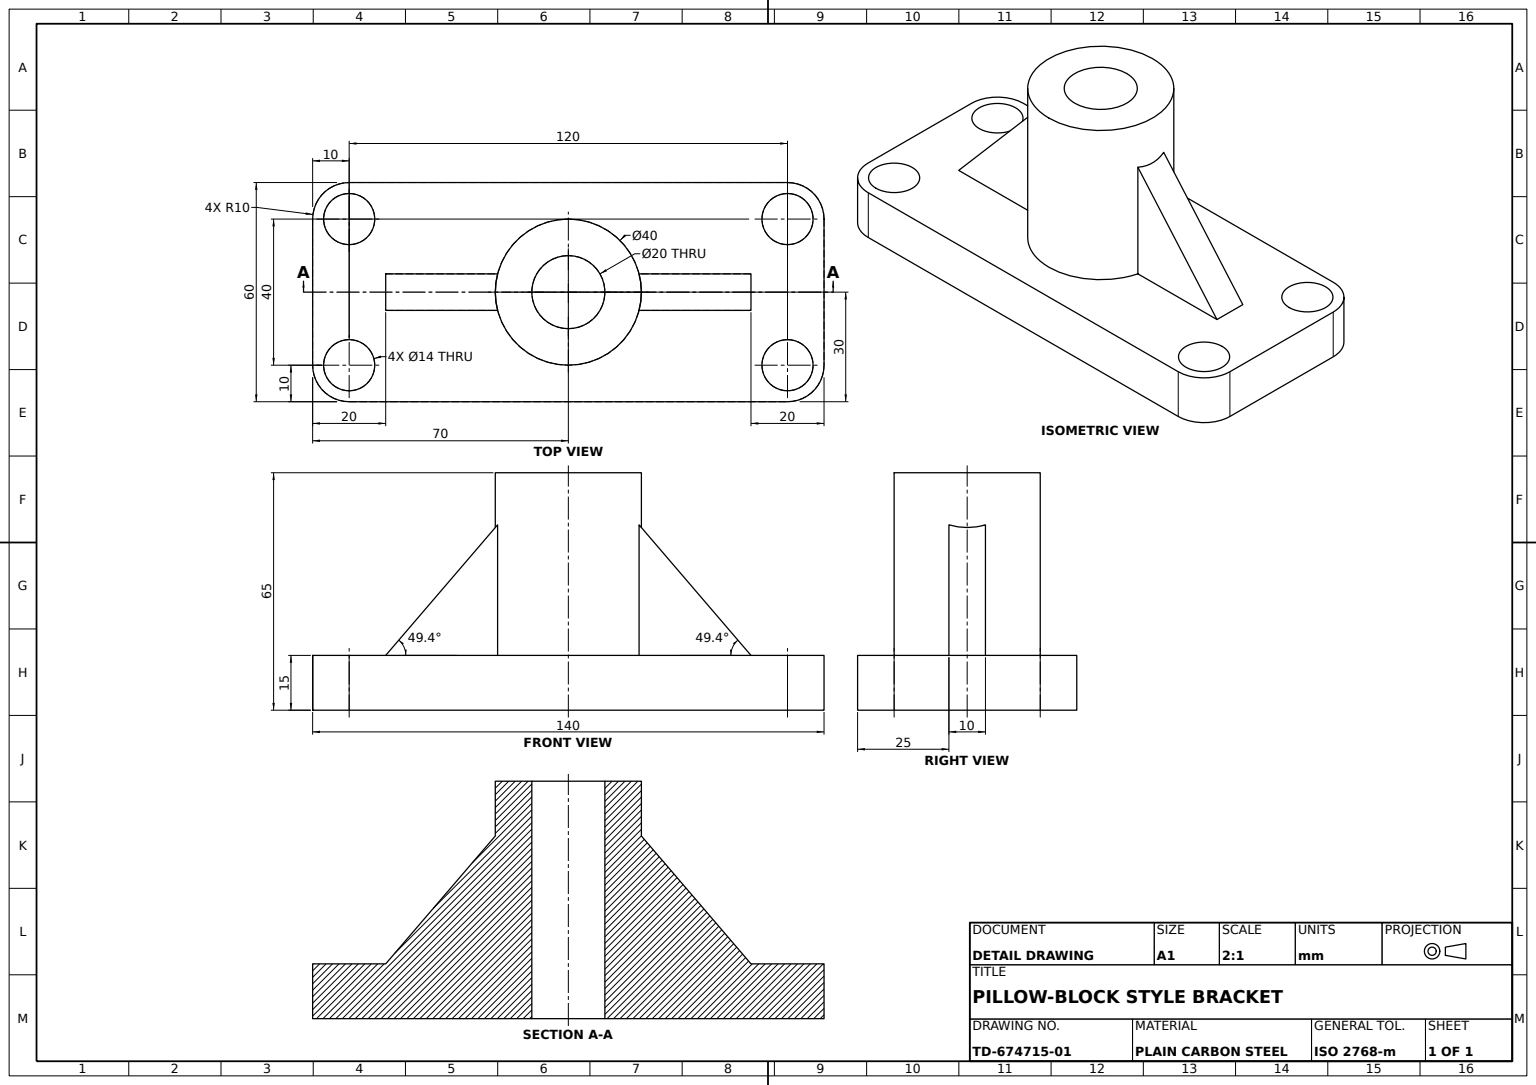
SolidWorks part; units mm, degrees
material "Plain Carbon Steel"
ref_plane "Front Plane" through (0, 0, 0) normal (0, 0, 1) x (1, 0, 0)
ref_plane "Top Plane" through (0, 0, 0) normal (0, 1, 0) x (1, 0, 0)
ref_plane "Right Plane" through (0, 0, 0) normal (1, 0, 0) x (0, 0, -1)
sketch "Base Plate Profile" plane through (0, 0, 0) normal (0, 1, 0) x (1, 0, 0)
  line L0 (70, 20) -> (70, -20)
  line L2 (60, 30) -> (-60, 30)
  line L3 (-70, 20) -> (-70, -20)
  line L4 (-60, -30) -> (60, -30)
  arc A0 (-60, 30) -> (-70, 20) centre (-60, 20) ccw
  arc A1 (-70, -20) -> (-60, -30) centre (-60, -20) ccw
  arc A2 (60, -30) -> (70, -20) centre (60, -20) ccw
  arc A3 (70, 20) -> (60, 30) centre (60, 20) ccw
  circle A4 centre (-60, 20) radius 5
  circle A5 centre (-60, 20) radius 7
  circle A6 centre (60, 20) radius 5
  circle A7 centre (60, 20) radius 7
  circle A8 centre (60, -20) radius 7
  circle A9 centre (60, -20) radius 5
  circle A10 centre (-60, -20) radius 5
  circle A11 centre (-60, -20) radius 7
  dimension "D1" = 10
  dimension "D2" = 120
  dimension "D6" = 14
  dimension "D7" = 10
  dimension "D8" = 14
  dimension "D9" = 10
  dimension "D10" = 14
  dimension "D11" = 10
  dimension "D12" = 14
  dimension "D13" = 10
  dimension "D3" = 30
  dimension "D4" = 30
  dimension "D5" = 70
extrude "Base Plate with Mounting Holes" add sketch "Base Plate Profile" along normal blind 15 contours L0 A3 L2 A0 L3 A1 L4 A2 A8 A5 A7 A11
sketch "Bearing Boss Profile" plane through (0, 15, 0) normal (0, 1, 0) x (1, 0, 0)
  circle A0 centre (0, 0) radius 20
  dimension "D1" = 40
extrude "Bearing Boss" add sketch "Bearing Boss Profile" along normal blind 50
sketch "Bore Profile" plane through (0, 65, 0) normal (0, 1, 0) x (1, 0, 0)
  circle A0 centre (0, 0) radius 10
  dimension "D1" = 20
extrude "Bearing Bore" cut sketch "Bore Profile" against normal blind 243
sketch "Support Rib Profile" plane through (0, 0, 0) normal (0, 0, 1) x (1, 0, 0)
  line L1 (-60, 15) -> (60, 15) construction
  line L3 (20, 15) -> (20, 65) construction
  line L4 (20, 50) -> (50, 15)
  dimension "D1" = 30
  dimension "D2" = 35
rib "Support Rib" sketch "Support Rib Profile" sketch "Support Rib Profile" thickness 10 extrusion direction parallel to sketch draft on no parameters "D1"=10
mirror "Support Rib Mirror" about plane through (0, 0, 0) normal (1, 0, 0) of "Support Rib"
